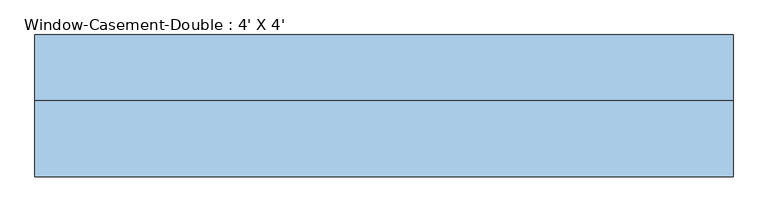
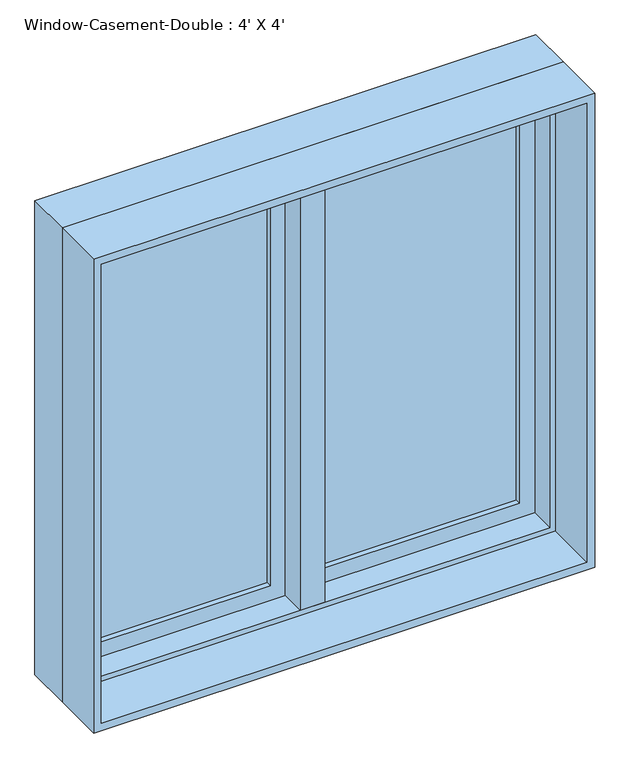
"""IFC4 building model written with IfcOpenShell, lengths in millimetres: window geometry, Window-Casement-Double : 4' X 4'."""

from ifc_helpers import new_model, si_unit, frame, origin, place, context, project, spatial, polyline, outline, extrude, faceted_brep, source, transform, mapped, element, save


def window_casement_double_4_x_4_9200f5ac(model_context):
    return source(origin(), model_context, "Body", "SolidModel", [
        faceted_brep([(577.85, 82.55, 2101.85), (577.85, 19.05, 2101.85), (-577.85, 19.05, 2101.85), (-577.85, 82.55, 2101.85), (596.9, 133.35, 2120.9), (596.9, 82.55, 2120.9), (-596.9, 82.55, 2120.9), (-596.9, 133.35, 2120.9), (609.6, 19.05, 2133.6), (609.6, 133.35, 2133.6), (-609.6, 133.35, 2133.6), (-609.6, 19.05, 2133.6), (-577.85, 19.05, 946.15), (-577.85, 82.55, 946.15), (-596.9, 82.55, 927.1), (-596.9, 133.35, 927.1), (-609.6, 133.35, 914.4), (-609.6, 19.05, 914.4), (577.85, 19.05, 946.15), (577.85, 82.55, 946.15), (596.9, 82.55, 927.1), (596.9, 133.35, 927.1), (609.6, 133.35, 914.4), (609.6, 19.05, 914.4)], [[[0, 1, 2, 3]], [[4, 5, 6, 7]], [[8, 9, 10, 11]], [[3, 2, 12, 13]], [[7, 6, 14, 15]], [[11, 10, 16, 17]], [[13, 12, 18, 19]], [[15, 14, 20, 21]], [[17, 16, 22, 23]], [[11, 17, 23, 8], [1, 18, 12, 2]], [[19, 18, 1, 0]], [[5, 20, 14, 6], [3, 13, 19, 0]], [[21, 20, 5, 4]], [[23, 22, 9, 8]], [[9, 22, 16, 10], [7, 15, 21, 4]]]),
        extrude(outline(polyline([(2133.6, -609.6), (914.4, -609.6), (914.4, 609.6), (2133.6, 609.6), (2133.6, -609.6)]), holes=[polyline([(2114.55, 590.55), (933.45, 590.55), (933.45, -590.55), (2114.55, -590.55), (2114.55, 590.55)])]), frame((0.0, -114.3, 0.0), z_axis=(0.0, 1.0, 0.0), x_axis=(0.0, 0.0, 1.0)), (0.0, 0.0, 1.0), 133.35),
        extrude(outline(polyline([(927.1, 596.9), (2120.9, 596.9), (2120.9, 9.525), (927.1, 9.525), (927.1, 596.9)]), holes=[polyline([(984.25, 66.675), (2063.75, 66.675), (2063.75, 539.75), (984.25, 539.75), (984.25, 66.675)])]), frame((0.0, 82.55, 0.0), z_axis=(0.0, 1.0, 0.0), x_axis=(0.0, 0.0, 1.0)), (0.0, 0.0, 1.0), 44.45),
        extrude(outline(polyline([(2120.9, -596.9), (927.1, -596.9), (927.1, -9.525), (2120.9, -9.525), (2120.9, -596.9)]), holes=[polyline([(2063.75, -66.675), (984.25, -66.675), (984.25, -539.75), (2063.75, -539.75), (2063.75, -66.675)])]), frame((0.0, 82.55, 0.0), z_axis=(0.0, 1.0, 0.0), x_axis=(0.0, 0.0, 1.0)), (0.0, 0.0, 1.0), 44.45),
        extrude(outline(polyline([(539.75, 114.3), (539.75, 107.95), (66.675, 107.95), (66.675, 114.3), (539.75, 114.3)])), frame((0.0, 0.0, 984.25), z_axis=(0.0, 0.0, 1.0), x_axis=(1.0, 0.0, 0.0)), (0.0, 0.0, 1.0), 1079.5),
        extrude(outline(polyline([(66.675, 95.25), (66.675, 101.6), (539.75, 101.6), (539.75, 95.25), (66.675, 95.25)])), frame((0.0, 0.0, 984.25), z_axis=(0.0, 0.0, 1.0), x_axis=(1.0, 0.0, 0.0)), (0.0, 0.0, 1.0), 1079.5),
        extrude(outline(polyline([(-66.675, 114.3), (-66.675, 107.95), (-539.75, 107.95), (-539.75, 114.3), (-66.675, 114.3)])), frame((0.0, 0.0, 984.25), z_axis=(0.0, 0.0, 1.0), x_axis=(1.0, 0.0, 0.0)), (0.0, 0.0, 1.0), 1079.5),
        extrude(outline(polyline([(-539.75, 95.25), (-539.75, 101.6), (-66.675, 101.6), (-66.675, 95.25), (-539.75, 95.25)])), frame((0.0, 0.0, 984.25), z_axis=(0.0, 0.0, 1.0), x_axis=(1.0, 0.0, 0.0)), (0.0, 0.0, 1.0), 1079.5),
        faceted_brep([(9.525, 133.35, 2120.9), (-9.525, 133.35, 2120.9), (-9.525, 82.55, 2120.9), (9.525, 82.55, 2120.9), (9.525, 133.35, 927.1), (9.525, 82.55, 927.1), (-9.525, 82.55, 927.1), (-9.525, 133.35, 927.1), (-9.525, 82.55, 946.15), (-9.525, 82.55, 2101.85), (-30.1625, 82.55, 946.15), (-30.1625, 82.55, 2101.85), (-30.1625, 19.05, 946.15), (-30.1625, 19.05, 2101.85), (30.1625, 19.05, 946.15), (30.1625, 19.05, 2101.85), (30.1625, 82.55, 946.15), (30.1625, 82.55, 2101.85), (9.525, 82.55, 946.15), (9.525, 82.55, 2101.85)], [[[0, 1, 2, 3]], [[4, 5, 6, 7]], [[1, 0, 4, 7]], [[2, 1, 7, 6, 8, 9]], [[9, 8, 10, 11]], [[11, 10, 12, 13]], [[13, 12, 14, 15]], [[15, 14, 16, 17]], [[17, 16, 18, 19]], [[0, 3, 19, 18, 5, 4]], [[18, 8, 6, 5]], [[9, 19, 3, 2]], [[8, 18, 16, 14, 12, 10]], [[19, 9, 11, 13, 15, 17]]]),
    ])


if __name__ == "__main__":
    model = new_model("IFC4")
    model_context = context("Model", 3, world=origin())
    ifc_project = project(units=[si_unit("LENGTHUNIT", "METRE", prefix="MILLI")], contexts=[model_context])
    site = spatial("IfcSite", under=ifc_project)
    building = spatial("IfcBuilding", under=site)
    placement = place(None, origin())
    window_casement_double_4_x_4_shape = window_casement_double_4_x_4_9200f5ac(model_context)
    element("IfcWindow", 1, ObjectType="Window-Casement-Double : 4' X 4'", at=placement, inside=building, context=model_context, shape_type="MappedRepresentation", body=[
        mapped(window_casement_double_4_x_4_shape, transform((0.0, 0.0, 0.0), x_axis=(1.0, 0.0, 0.0), y_axis=(0.0, 1.0, 0.0), z_axis=(0.0, 0.0, 1.0))),
    ])
    save(model, "model.ifc")

# Revit data of these elements
# Type "Window-Casement-Double : 4' X 4'"
#   Type Mark = "19"
#   Fire Rating = "0.5h"
#   Assembly Code = "B2020100"
#   Analytic Construction = "Double glazing - domestic"
#   Frame Extension [instance default] = 0' - 0 1/4"
#   Window Inset [instance default] = 0' - 0"
#   Wall Thickness [instance default] = 0' - 6"
#   Interior Wall Closure [instance default] = 0' - 2 1/4"
#   Half Width = 2' - 0"
#   Visual Light Transmittance = 0.81
#   Thermal Resistance (R) = 1.8146 (h·ft²·°F)/BTU
#   Solar Heat Gain Coefficient = 0.76
#   Rough Width = 4' - 0 1/2"
#   Rough Height = 4' - 0 1/2"
#   Height = 4' - 0"
#   Heat Transfer Coefficient (U) = 0.5511 BTU/(h·ft²·°F)
#   Exterior Wall Closure [instance default] = 0' - 1 1/4"
#   Extension Jamb [instance default] = 0' - 2 1/4"
#   Default Sill Height = 3' - 0"
#   Width = 4' - 0"
#   Muntin Visibility = yes
#   Interior Trim Visibility [instance default] = yes
#   Exterior Trim Visibility [instance default] = yes
#   Extension Jamb Visibility [instance default] = yes
#   Interior Trim Material = Wood - Stained
#   Muntin Pattern = Muntin Pattern_2x2 : Muntin Pattern_2x2
#   Interior Trim = Trim-Window-Interior-Flat : Picture Frame
#   Interior Frame Material = Wood - Stained
#   Glass Panel Material = Glass
#   Exterior Trim Material = Clad - White
#   Exterior Trim = Trim-Window-Exterior-Flat : with Sill
#   Exterior Frame Material = Clad - White
#   Wall Closure = (empty or 0)
# Element 1 (IfcWindow, "Window-Casement-Double : 4' X 4'")
#   Wall Thickness = 0' - 9"
#   Extension Jamb = 0' - 5 1/4"
#   Materials on its faces: "Wood - Stained", "Glass", "Clad - White"
# Materials
#   "Wood - Stained": class "Wood", colour RGB 224 178 126, transparency 0, Cost = 0
#   "Glass": class "Glass", colour RGB 0 128 192, transparency 0.75, Description = "Soda Lime Glass", Cost = 0
#   "Clad - White": class "Wood", colour RGB 242 242 238, transparency 0, Cost = 0
